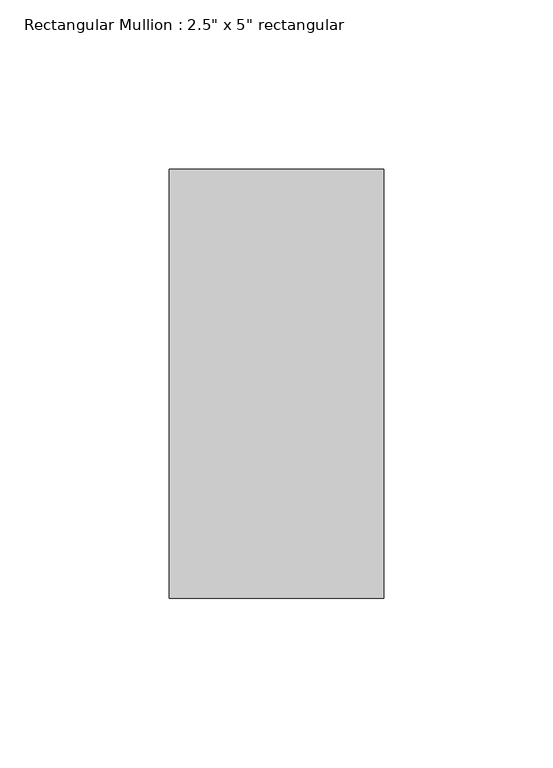
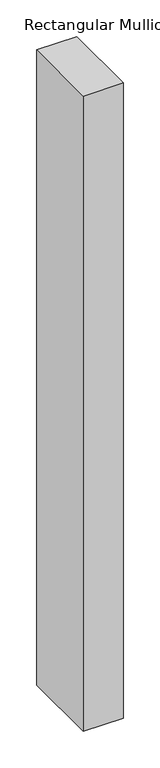
"""IFC4 building model written with IfcOpenShell, lengths in millimetres: member geometry."""

from ifc_helpers import new_model, si_unit, frame, origin, place, context, project, spatial, polyline, outline, extrude, source, transform, mapped, element, save


def member_d13a5c2f(model_context):
    return source(origin(), model_context, "Body", "SweptSolid", [
        extrude(outline(polyline([(0.0, 63.5), (0.0, -63.5), (-63.5, -63.5), (-63.5, 63.5), (0.0, 63.5)])), frame((0.0, 0.0, -1060.45), z_axis=(0.0, 0.0, 1.0), x_axis=(1.0, 0.0, 0.0)), (0.0, 0.0, 1.0), 1060.45),
    ])


if __name__ == "__main__":
    model = new_model("IFC4")
    model_context = context("Model", 3, world=origin())
    ifc_project = project(units=[si_unit("LENGTHUNIT", "METRE", prefix="MILLI")], contexts=[model_context])
    site = spatial("IfcSite", under=ifc_project)
    building = spatial("IfcBuilding", under=site)
    placement = place(None, origin())
    member_shape = member_d13a5c2f(model_context)
    element("IfcMember", 1, ObjectType="Rectangular Mullion : 2.5\" x 5\" rectangular", at=placement, inside=building, context=model_context, shape_type="MappedRepresentation", body=[
        mapped(member_shape, transform((0.0, 0.0, 0.0), x_axis=(1.0, 0.0, 0.0), y_axis=(0.0, 1.0, 0.0), z_axis=(0.0, 0.0, 1.0))),
    ])
    save(model, "model.ifc")

# Revit data of these elements
# Type "Rectangular Mullion : 2.5\" x 5\" rectangular"
#   built-in parameter 1007304 = 0.416667 (stored number, unit not read)
#   built-in parameter 1007301 = 0.104167 (stored number, unit not read)
#   built-in parameter 1007300 = 0.104167 (stored number, unit not read)
# Element 1 (IfcMember, "Rectangular Mullion : 2.5\" x 5\" rectangular")
#   Materials on its faces: "mullions"
# Materials
#   "mullions": class "Generic", colour RGB 120 120 120, transparency 0, Cost = 0
